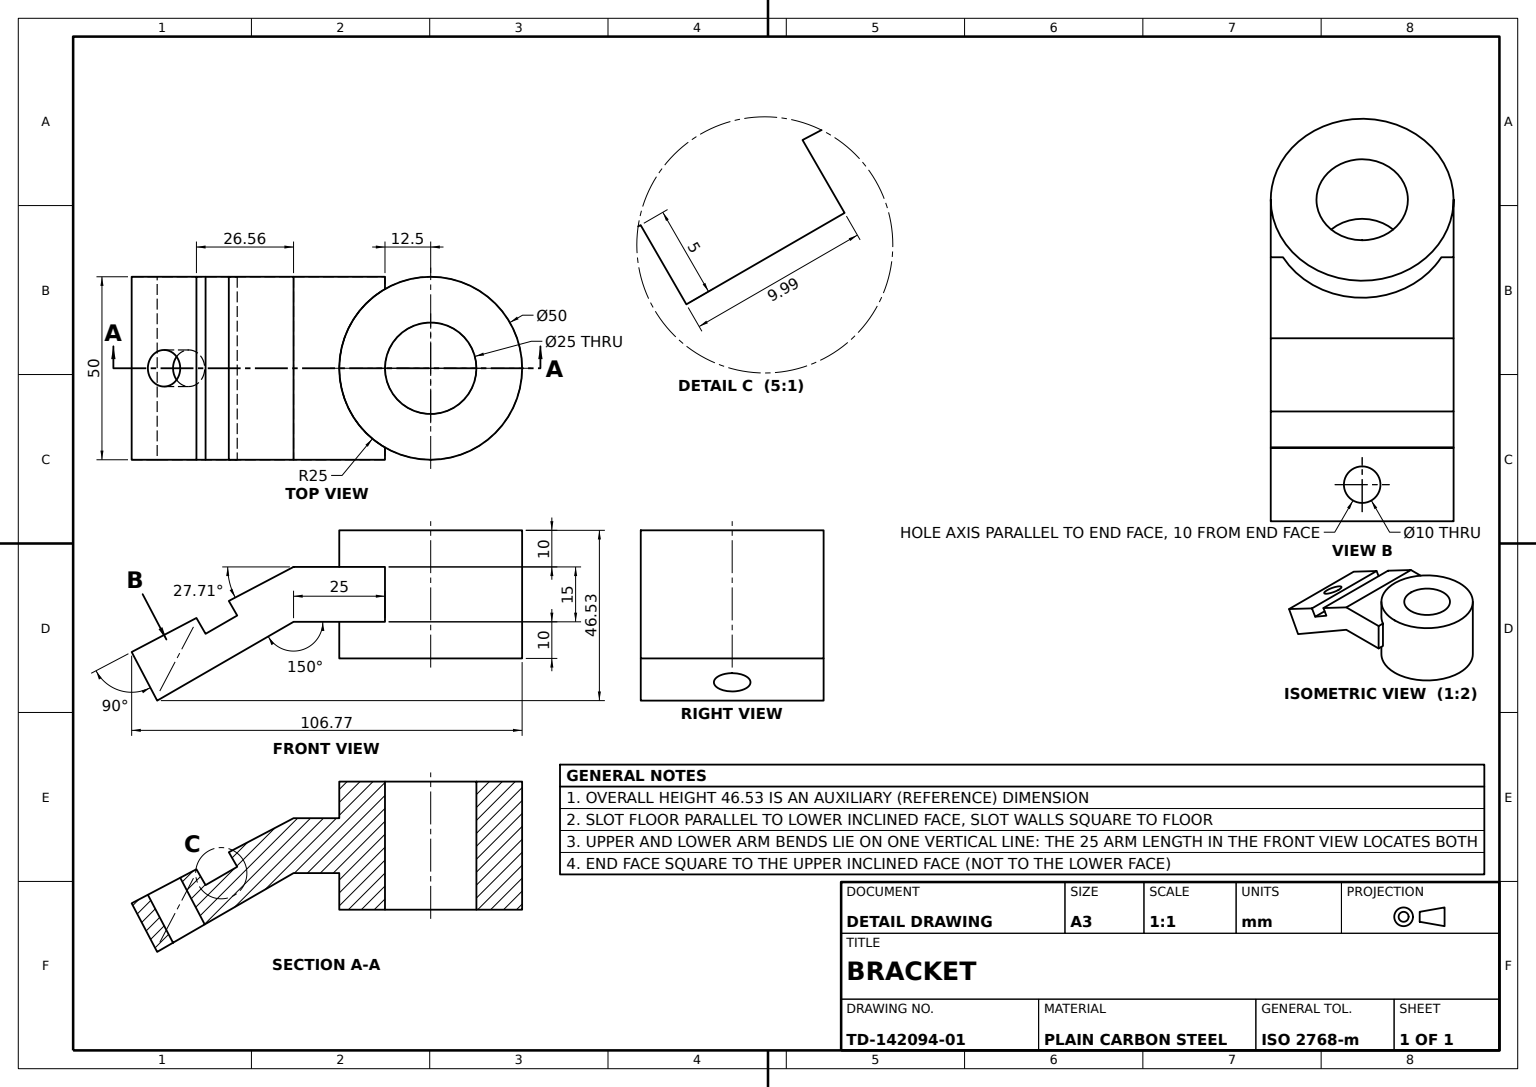
from build123d import *

# Parameters (mm, degrees)
BASE_BLOCK_DEPTH       = 25
CYLINDER_BOSS_SKETCH_R = 25
CYLINDER_BOSS_50_DEPTH = 25
WEB_START              = 10
WEB_BOSS_DEPTH         = 10
BORE_SKETCH_R          = 12.5
BORE_25_DEPTH          = 82.533502
T_SLOT_CUT_DEPTH       = 90.009618
HOLE_SKETCH_R          = 5
HOLE_10_DEPTH          = 77.495661


with BuildPart() as part:
    # Base Profile Sketch → Base Block (new, symmetric)
    with BuildSketch(Plane.XY):
        Polygon((0, 0), (-25, 0), (-62.290509, -21.529686), (-69.265518, -8.25003), (-25, 15), (0, 15), align=None)
    extrude(amount=BASE_BLOCK_DEPTH, both=True)

    # Cylinder Boss Sketch → Cylinder Boss Ø50 (add)
    with BuildSketch(Plane(origin=(0, 0, 0), x_dir=(1, 0, 0), z_dir=(0, 1, 0))):
        with Locations(Location((12.5, 0, 0), (0, 0, 120))):
            Circle(CYLINDER_BOSS_SKETCH_R)
    extrude(amount=CYLINDER_BOSS_50_DEPTH)

    # Web Boss Sketch → Web Boss (add)
    with BuildSketch(Plane.XZ.offset(WEB_START)):
        with BuildLine():
            ThreePointArc((0, 21.650635), (-12.5, 0), (0, -21.650635))
            ThreePointArc((0, -21.650635), (25, -21.650635), (37.5, 0))
            ThreePointArc((37.5, 0), (25, 21.650635), (0, 21.650635))
        make_face()
    extrude(amount=-WEB_BOSS_DEPTH)

    # Bore Sketch → Bore Ø25 (cut, through all)
    with BuildSketch(Plane.XZ.offset(10)):
        with Locations((12.5, 0)):
            Circle(BORE_SKETCH_R)
    extrude(amount=-BORE_25_DEPTH, mode=Mode.SUBTRACT)

    # T-Slot Sketch → T-Slot Cut (cut, through all)
    with BuildSketch(Plane.XY.offset(25)):
        Polygon((-42.70267, 5.701846), (-51.555777, 1.051838), (-49.055777, -3.278289), (-40.402434, 1.717721), align=None)
    extrude(amount=-T_SLOT_CUT_DEPTH, mode=Mode.SUBTRACT)

    # Hole Sketch → Hole Ø10 (cut, through all)
    with BuildSketch(Plane(origin=(-11.580687, 22.048363, 0), x_dir=(0.8853103641838149, 0.4650006011487738, 0), z_dir=(-0.4650006011487738, 0.8853103641838149, 0))):
        with Locations(Location((-55.155754, 0, 0), (0, 0, 180))):
            Circle(HOLE_SKETCH_R)
    extrude(amount=-HOLE_10_DEPTH, mode=Mode.SUBTRACT)


solid = part.part
